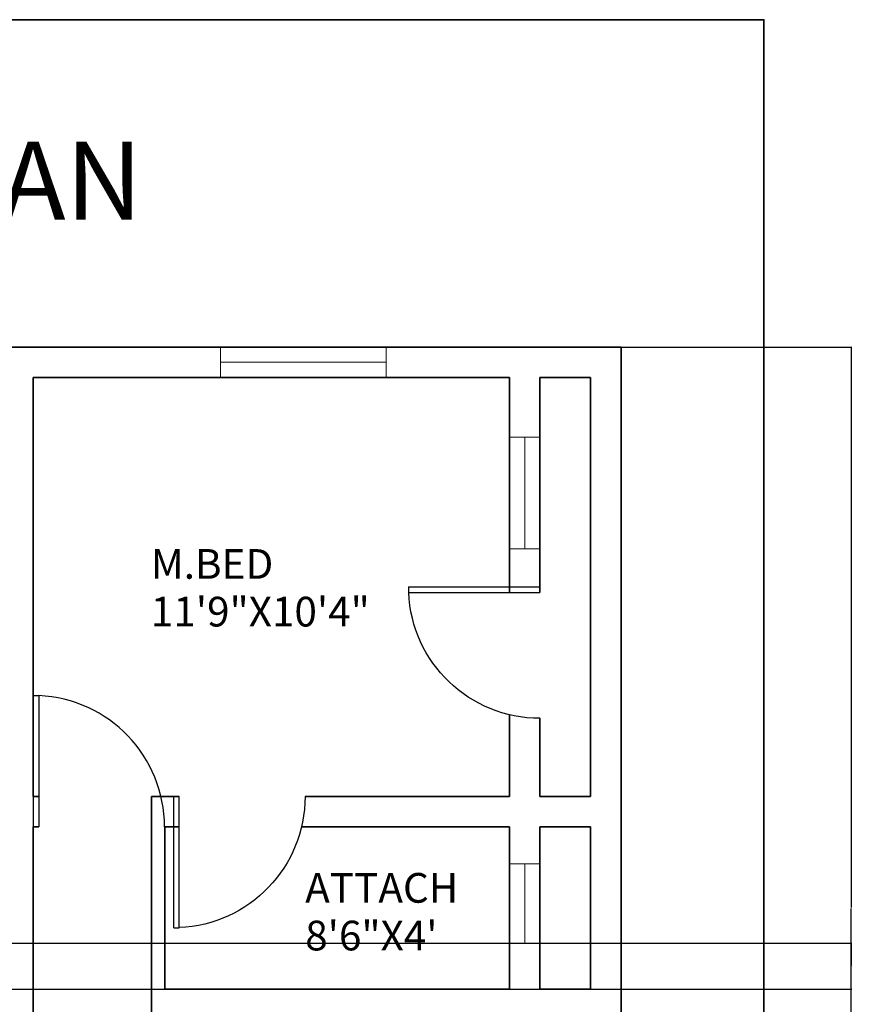
# Model space of a CAD drawing. Units: feet. Extents: x 100807 to 101423, y 154875 to 156331.
# Tile 8 of 8: x 101176 to 101423, y 156040 to 156331. Entities that reach past the tile are written whole.
import ezdxf

# ---------------------------------------------------------------- set-up
doc = ezdxf.new("R2010")
doc.units = ezdxf.units.FT
for name, color, linetype, lineweight in [('A-ANNO-DIMS', 2, 'Continuous', 18), ('A-ANNO-TITL', 7, 'Continuous', 35), ('A-ANNO-TTLB', 7, 'Continuous', 35), ('A-AREA-IDEN', 7, 'Continuous', 25), ('A-DOOR', 4, 'Continuous', 25), ('A-GLAZ', 4, 'Continuous', 18), ('A-WALL', 7, 'Continuous', 35)]:
    doc.layers.add(name, color=color, linetype=linetype, lineweight=lineweight)
doc.styles.get("Standard").update_dxf_attribs({"font": 'arial.ttf'})
doc.dimstyles.get("Standard").update_dxf_attribs({"dimtxt": 0.18, "dimasz": 0.18, "dimexe": 0.18, "dimexo": 0.0625, "dimgap": 0.09, "dimtad": 0, "dimtih": 1, "dimtoh": 1, "dimdec": 4, "dimzin": 0, "dimdsep": 46, "dimtxsty": 'Standard', "dimcen": 0.09, "dimadec": 0, "dimazin": 0, "dimtfac": 1, "dimtdec": 4, "dimtofl": 0, "dimtmove": 0, "dimatfit": 3, "dimfxl": 1, "dimtolj": 1, "dimtzin": 0, "dimarcsym": 0})

# ---------------------------------------------------------------- blocks, each defined once
blk = doc.blocks.new('DR-36')
for p, q in [((0, 36), (0, 0)), ((0, 36), (1.5, 36)), ((1.5, 36), (1.5, 0)), ((0, 0), (1.5, 0))]:
    blk.add_line(p, q)
blk.add_arc((0, 0), 36, 0, 87.6141)
blk = doc.blocks.new('WIN-BATH-SIDE')
for p, q in [((0, 23.54), (9, 23.54)), ((4.5, 23.54), (4.5, 0)), ((0, 0), (9, 0))]:
    blk.add_line(p, q)
blk = doc.blocks.new('WIN-MBED-SIDE')
for p, q in [((0, 33.08), (9, 33.08)), ((4.5, 33.08), (4.5, 0)), ((0, 0), (9, 0))]:
    blk.add_line(p, q)
blk = doc.blocks.new('*D41')
at = {"layer": 'A-ANNO-DIMS', "color": 0, "lineweight": -2, "transparency": 16777216}
for p, q in [((101354.22, 156234.58), (101422.49, 156234.58)), ((101422.31, 156234.4), (101422.31, 156068.76)), ((101422.31, 155902.76), (101422.31, 156068.4)), ((101354.22, 155902.58), (101422.49, 155902.58))]:
    blk.add_line(p, q, dxfattribs=at)
at = {"layer": 'A-ANNO-DIMS', "color": 0, "transparency": 16777216}
for points in [[(101422.28, 156234.4), (101422.34, 156234.4), (101422.31, 156234.58)], [(101422.28, 155902.76), (101422.34, 155902.76), (101422.31, 155902.58)]]:
    blk.add_solid(points, dxfattribs=at)
at = {"layer": 'Defpoints', "color": 0, "transparency": 16777216}
for p in [(101354.16, 156234.58), (101422.31, 156234.58), (101354.16, 155902.58)]:
    blk.add_point(p, dxfattribs=at)
at = {"layer": 'A-ANNO-DIMS', "color": 0, "transparency": 16777216, "insert": (101422.31, 156068.58), "char_height": 0.18, "attachment_point": 5}
blk.add_mtext('\\A1;332', dxfattribs=at)
blk = doc.blocks.new('*D55')
at = {"layer": 'A-ANNO-DIMS', "color": 0, "lineweight": -2, "transparency": 16777216}
for p, q in [((100908.22, 156058.13), (101422.49, 156058.13)), ((101422.31, 156057.95), (101422.31, 156051.53)), ((101422.31, 156044.76), (101422.31, 156051.17)), ((100908.22, 156044.58), (101422.49, 156044.58))]:
    blk.add_line(p, q, dxfattribs=at)
at = {"layer": 'A-ANNO-DIMS', "color": 0, "transparency": 16777216}
for points in [[(101422.28, 156057.95), (101422.34, 156057.95), (101422.31, 156058.13)], [(101422.28, 156044.76), (101422.34, 156044.76), (101422.31, 156044.58)]]:
    blk.add_solid(points, dxfattribs=at)
at = {"layer": 'Defpoints', "color": 0, "transparency": 16777216}
for p in [(100908.16, 156058.13), (101422.31, 156058.13), (100908.16, 156044.58)]:
    blk.add_point(p, dxfattribs=at)
at = {"layer": 'A-ANNO-DIMS', "color": 0, "transparency": 16777216, "insert": (101422.31, 156051.35), "char_height": 0.18, "attachment_point": 5}
blk.add_mtext('\\A1;13.55', dxfattribs=at)

msp = doc.modelspace()

# ---------------------------------------------------------------- linework, layer by layer
at = {"layer": 'A-ANNO-TTLB'}
msp.add_lwpolyline([(100830.3877, 156331.4447), (101396.4426, 156331.4447), (101396.4426, 154875.4601), (100830.3877, 154875.4601)], close=True, dxfattribs=at)
at = {"layer": 'A-GLAZ'}
for p, q in [((101235.6093, 156234.5777), (101235.6093, 156225.5777)), ((101284.6543, 156234.5777), (101284.6543, 156225.5777)), ((101235.6093, 156230.0777), (101284.6543, 156230.0777))]:
    msp.add_line(p, q, dxfattribs=at)
at = {"layer": 'A-WALL'}
for p, q in [((101354.1564, 156234.5777), (101171.1564, 156234.5777)), ((101354.1564, 156035.5777), (101354.1564, 156234.5777)), ((101321.1564, 156225.5777), (101180.1564, 156225.5777)), ((101180.1564, 156225.5777), (101180.1564, 156101.5777)), ((101321.1564, 156161.9582), (101321.1564, 156225.5777)), ((101345.1564, 156225.5777), (101330.1564, 156225.5777)), ((101330.1564, 156161.9582), (101330.1564, 156225.5777)), ((101345.1564, 156101.5777), (101345.1564, 156225.5777)), ((101321.1564, 156101.5777), (101321.1564, 156125.7659)), ((101330.1564, 156101.5777), (101330.1564, 156124.7095)), ((101180.1564, 156101.5777), (101181.7759, 156101.5777)), ((101215.1564, 156101.5777), (101223.3792, 156101.5777)), ((101215.1564, 156092.5777), (101215.1564, 156101.5777)), ((101260.6279, 156101.5777), (101321.1564, 156101.5777)), ((101330.1564, 156101.5777), (101345.1564, 156101.5777)), ((101180.1564, 156092.5777), (101180.1564, 156021.9594)), ((101180.1564, 156092.5777), (101181.7759, 156092.5777)), ((101215.1564, 156044.5777), (101215.1564, 156092.5777)), ((101215.1564, 155945.4459), (101215.1564, 156092.5777)), ((101219.1564, 156092.5777), (101223.3792, 156092.5777)), ((101219.1564, 156044.5777), (101219.1564, 156092.5777)), ((101259.5661, 156092.5777), (101321.1564, 156092.5777)), ((101321.1564, 156092.5777), (101321.1564, 156044.5777)), ((101330.1564, 156092.5777), (101345.1564, 156092.5777)), ((101330.1564, 156092.5777), (101330.1564, 156044.5777)), ((101345.1564, 156044.5777), (101345.1564, 156092.5777)), ((101321.1564, 156044.5777), (101219.1564, 156044.5777)), ((101345.1564, 156044.5777), (101330.1564, 156044.5777))]:
    msp.add_line(p, q, dxfattribs=at)

# ---------------------------------------------------------------- block references
at = {"layer": 'A-DOOR', "xscale": -1.079672442471032, "yscale": 1.079672442471032, "zscale": 1.079672442471032}
for p, rotation in [((101330.1564, 156163.5777), 90), ((101221.7597, 156101.6007), 180)]:
    msp.add_blockref('DR-36', p, dxfattribs=dict(at, rotation=rotation))
at = {"layer": 'A-DOOR', "xscale": 1.079672442471032, "yscale": 1.079672442471032, "zscale": 1.079672442471032}
msp.add_blockref('DR-36', (101180.1564, 156092.5777), dxfattribs=at)
at = {"layer": 'A-GLAZ', "rotation": 180}
msp.add_blockref('WIN-MBED-SIDE', (101330.1564, 156207.9304), dxfattribs=at)
at = {"layer": 'A-GLAZ'}
msp.add_blockref('WIN-BATH-SIDE', (101321.1564, 156058.1276), dxfattribs=at)

# ---------------------------------------------------------------- texts
at = {"layer": 'A-ANNO-DIMS'}
for s, height, p in [('11\'9"X10\'4"', 8.788223, (101214.976, 156151.8819)), ('8\'6"X4\'', 8.78822, (101260.6646, 156056.0266))]:
    msp.add_text(s, height=height, dxfattribs=at).set_placement(p)
at = {"layer": 'A-ANNO-TITL'}
msp.add_text('FLOOR PLAN', height=23.08638, dxfattribs=at).set_placement((101025.2804, 156272.2968))
at = {"layer": 'A-AREA-IDEN'}
for s, p in [('M.BED', (101214.976, 156165.9994)), ('ATTACH', (101260.6646, 156070.1441))]:
    msp.add_text(s, height=8.78822, dxfattribs=at).set_placement(p)

# ---------------------------------------------------------------- dimensions: what is measured, and where the dimension line sits
at = {"layer": 'A-ANNO-DIMS'}
for base, p1, p2, override, picture, middle in [((101422.3064, 156234.5777), (101354.1564, 155902.5777), (101354.1564, 156234.5777), {"dimdec": 0, "dimlfac": 1, "dimrnd": 0, "dimzin": 0, "dimdsep": 46, "dimlunit": 2}, '*D41', (101422.3064, 156068.5777)), ((101422.3064, 156058.1276), (100908.1564, 156044.5777), (100908.1564, 156058.1276), {"dimdec": 2, "dimlfac": 1, "dimrnd": 0, "dimzin": 0, "dimdsep": 46, "dimlunit": 2}, '*D55', (101422.3064, 156051.3527))]:
    dim = msp.add_linear_dim(base=base, p1=p1, p2=p2, angle=90, dimstyle='Standard', override=override, dxfattribs=at)
    dim.commit()
    dim.dimension.update_dxf_attribs({"geometry": picture, "text_midpoint": middle})

doc.saveas('drawing.dxf')
